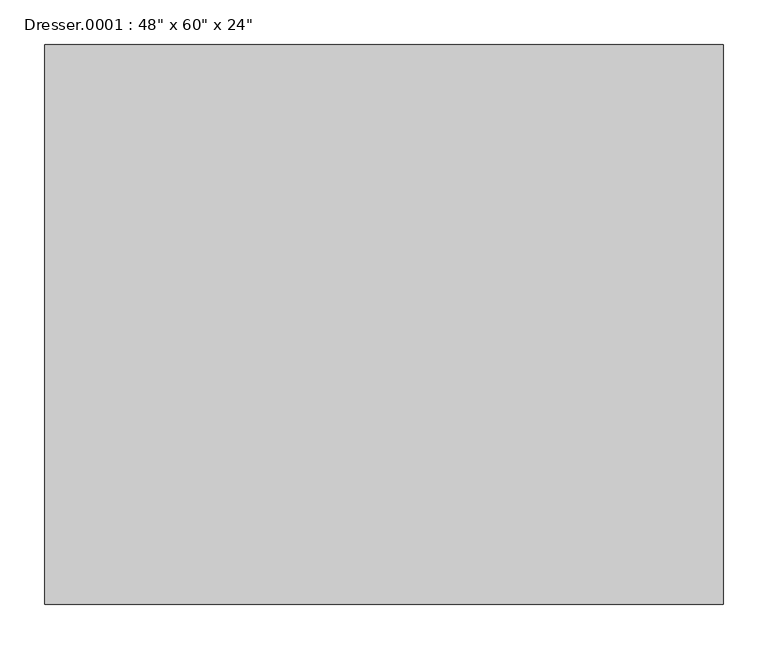
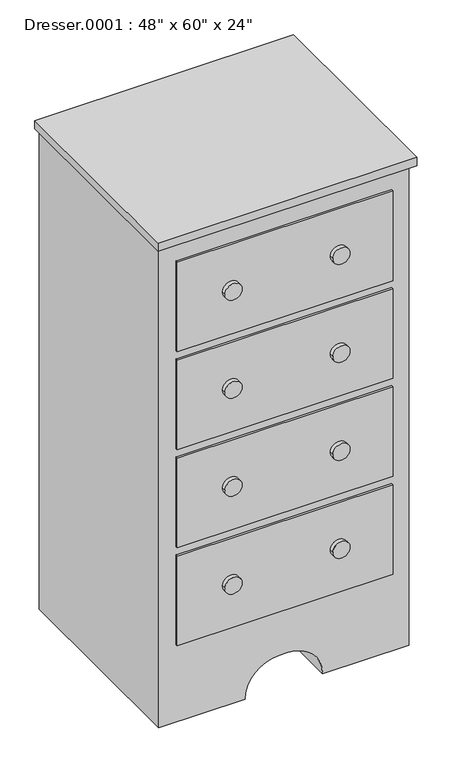
"""IFC4 building model written with IfcOpenShell, lengths in millimetres: furniture geometry."""

from ifc_helpers import new_model, si_unit, point, frame, frame_2d, origin, place, context, project, spatial, polyline, circle_curve, trimmed, segment, composite_curve, outline, extrude, source, transform, mapped, element, save


def furniture_08c10487(model_context):
    return source(origin(), model_context, "Body", "SweptSolid", [
        extrude(outline(polyline([(111.8067402, -58.3629541), (111.8067402, -687.0129541), (-650.1932598, -687.0129541), (-650.1932598, -58.3629541), (111.8067402, -58.3629541)])), frame((0.0, 0.0, 1498.6), z_axis=(0.0, 0.0, 1.0), x_axis=(1.0, 0.0, 0.0)), (0.0, 0.0, 1.0), 25.4),
        extrude(outline(composite_curve([segment(polyline([(0.0, 99.1067402), (1498.6, 99.1067402), (1498.6, -637.4932598), (0.0, -637.4932598), (0.0, -383.4932598)]), True, "CONTINUOUS"), segment(trimmed(circle_curve(frame_2d((0.0, -281.8932598)), 101.6), [point((0.0, -383.4932598))], [point((101.6, -281.8932598))], True, "CARTESIAN"), True, "CONTINUOUS"), segment(polyline([(101.6, -281.8932598), (101.6, -256.4932598)]), True, "CONTINUOUS"), segment(trimmed(circle_curve(frame_2d((0.0, -256.4932598)), 101.6), [point((101.6, -256.4932598))], [point((0.0, -154.8932598))], True, "CARTESIAN"), True, "CONTINUOUS"), segment(polyline([(0.0, -154.8932598), (0.0, 99.1067402)]), True, "CONTINUOUS")], self_intersect=False)), frame((0.0, -667.9629541, 0.0), z_axis=(0.0, 1.0, 0.0), x_axis=(0.0, 0.0, 1.0)), (0.0, 0.0, 1.0), 609.6),
        extrude(outline(composite_curve([segment(trimmed(circle_curve(frame_2d((1295.4, -110.4432598)), 25.4), [point((1295.4, -135.8432598))], [point((1295.4, -85.0432598))], False, "CARTESIAN"), True, "CONTINUOUS"), segment(trimmed(circle_curve(frame_2d((1295.4, -110.4432598)), 25.4), [point((1295.4, -85.0432598))], [point((1295.4, -135.8432598))], False, "CARTESIAN"), True, "CONTINUOUS")], self_intersect=False)), frame((0.0, -687.0129541, 0.0), z_axis=(0.0, 1.0, 0.0), x_axis=(0.0, 0.0, 1.0)), (0.0, 0.0, 1.0), 12.7),
        extrude(outline(composite_curve([segment(trimmed(circle_curve(frame_2d((990.6, -110.4432598)), 25.4), [point((990.6, -135.8432598))], [point((990.6, -85.0432598))], False, "CARTESIAN"), True, "CONTINUOUS"), segment(trimmed(circle_curve(frame_2d((990.6, -110.4432598)), 25.4), [point((990.6, -85.0432598))], [point((990.6, -135.8432598))], False, "CARTESIAN"), True, "CONTINUOUS")], self_intersect=False)), frame((0.0, -687.0129541, 0.0), z_axis=(0.0, 1.0, 0.0), x_axis=(0.0, 0.0, 1.0)), (0.0, 0.0, 1.0), 12.7),
        extrude(outline(composite_curve([segment(trimmed(circle_curve(frame_2d((685.8, -110.4432598)), 25.4), [point((685.8, -135.8432598))], [point((685.8, -85.0432598))], False, "CARTESIAN"), True, "CONTINUOUS"), segment(trimmed(circle_curve(frame_2d((685.8, -110.4432598)), 25.4), [point((685.8, -85.0432598))], [point((685.8, -135.8432598))], False, "CARTESIAN"), True, "CONTINUOUS")], self_intersect=False)), frame((0.0, -687.0129541, 0.0), z_axis=(0.0, 1.0, 0.0), x_axis=(0.0, 0.0, 1.0)), (0.0, 0.0, 1.0), 12.7),
        extrude(outline(composite_curve([segment(trimmed(circle_curve(frame_2d((381.0, -110.4432598)), 25.4), [point((381.0, -135.8432598))], [point((381.0, -85.0432598))], False, "CARTESIAN"), True, "CONTINUOUS"), segment(trimmed(circle_curve(frame_2d((381.0, -110.4432598)), 25.4), [point((381.0, -85.0432598))], [point((381.0, -135.8432598))], False, "CARTESIAN"), True, "CONTINUOUS")], self_intersect=False)), frame((0.0, -687.0129541, 0.0), z_axis=(0.0, 1.0, 0.0), x_axis=(0.0, 0.0, 1.0)), (0.0, 0.0, 1.0), 12.7),
        extrude(outline(composite_curve([segment(trimmed(circle_curve(frame_2d((381.0, -427.9432598)), 25.4), [point((381.0, -453.3432598))], [point((381.0, -402.5432598))], False, "CARTESIAN"), True, "CONTINUOUS"), segment(trimmed(circle_curve(frame_2d((381.0, -427.9432598)), 25.4), [point((381.0, -402.5432598))], [point((381.0, -453.3432598))], False, "CARTESIAN"), True, "CONTINUOUS")], self_intersect=False)), frame((0.0, -687.0129541, 0.0), z_axis=(0.0, 1.0, 0.0), x_axis=(0.0, 0.0, 1.0)), (0.0, 0.0, 1.0), 12.7),
        extrude(outline(composite_curve([segment(trimmed(circle_curve(frame_2d((685.8, -427.9432598)), 25.4), [point((685.8, -453.3432598))], [point((685.8, -402.5432598))], False, "CARTESIAN"), True, "CONTINUOUS"), segment(trimmed(circle_curve(frame_2d((685.8, -427.9432598)), 25.4), [point((685.8, -402.5432598))], [point((685.8, -453.3432598))], False, "CARTESIAN"), True, "CONTINUOUS")], self_intersect=False)), frame((0.0, -687.0129541, 0.0), z_axis=(0.0, 1.0, 0.0), x_axis=(0.0, 0.0, 1.0)), (0.0, 0.0, 1.0), 12.7),
        extrude(outline(composite_curve([segment(trimmed(circle_curve(frame_2d((990.6, -427.9432598)), 25.4), [point((990.6, -453.3432598))], [point((990.6, -402.5432598))], False, "CARTESIAN"), True, "CONTINUOUS"), segment(trimmed(circle_curve(frame_2d((990.6, -427.9432598)), 25.4), [point((990.6, -402.5432598))], [point((990.6, -453.3432598))], False, "CARTESIAN"), True, "CONTINUOUS")], self_intersect=False)), frame((0.0, -687.0129541, 0.0), z_axis=(0.0, 1.0, 0.0), x_axis=(0.0, 0.0, 1.0)), (0.0, 0.0, 1.0), 12.7),
        extrude(outline(composite_curve([segment(trimmed(circle_curve(frame_2d((1295.4, -427.9432598)), 25.4), [point((1295.4, -453.3432598))], [point((1295.4, -402.5432598))], False, "CARTESIAN"), True, "CONTINUOUS"), segment(trimmed(circle_curve(frame_2d((1295.4, -427.9432598)), 25.4), [point((1295.4, -402.5432598))], [point((1295.4, -453.3432598))], False, "CARTESIAN"), True, "CONTINUOUS")], self_intersect=False)), frame((0.0, -687.0129541, 0.0), z_axis=(0.0, 1.0, 0.0), x_axis=(0.0, 0.0, 1.0)), (0.0, 0.0, 1.0), 12.7),
        extrude(outline(polyline([(48.3067402, -674.3129541), (-586.6932598, -674.3129541), (-586.6932598, -667.9629541), (48.3067402, -667.9629541), (48.3067402, -674.3129541)])), frame((0.0, 0.0, 1155.7), z_axis=(0.0, 0.0, 1.0), x_axis=(1.0, 0.0, 0.0)), (0.0, 0.0, 1.0), 279.4),
        extrude(outline(polyline([(48.3067402, -674.3129541), (-586.6932598, -674.3129541), (-586.6932598, -667.9629541), (48.3067402, -667.9629541), (48.3067402, -674.3129541)])), frame((0.0, 0.0, 850.9), z_axis=(0.0, 0.0, 1.0), x_axis=(1.0, 0.0, 0.0)), (0.0, 0.0, 1.0), 279.4),
        extrude(outline(polyline([(48.3067402, -674.3129541), (-586.6932598, -674.3129541), (-586.6932598, -667.9629541), (48.3067402, -667.9629541), (48.3067402, -674.3129541)])), frame((0.0, 0.0, 546.1), z_axis=(0.0, 0.0, 1.0), x_axis=(1.0, 0.0, 0.0)), (0.0, 0.0, 1.0), 279.4),
        extrude(outline(polyline([(48.3067402, -674.3129541), (-586.6932598, -674.3129541), (-586.6932598, -667.9629541), (48.3067402, -667.9629541), (48.3067402, -674.3129541)])), frame((0.0, 0.0, 241.3), z_axis=(0.0, 0.0, 1.0), x_axis=(1.0, 0.0, 0.0)), (0.0, 0.0, 1.0), 279.4),
    ])


if __name__ == "__main__":
    model = new_model("IFC4")
    model_context = context("Model", 3, world=origin())
    ifc_project = project(units=[si_unit("LENGTHUNIT", "METRE", prefix="MILLI")], contexts=[model_context])
    site = spatial("IfcSite", under=ifc_project)
    building = spatial("IfcBuilding", under=site)
    placement = place(None, origin())
    furniture_shape = furniture_08c10487(model_context)
    element("IfcFurniture", 1, ObjectType="Dresser.0001 : 48\" x 60\" x 24\"", at=placement, inside=building, context=model_context, shape_type="MappedRepresentation", body=[
        mapped(furniture_shape, transform((0.0, 0.0, 0.0), x_axis=(1.0, 0.0, 0.0), y_axis=(0.0, 1.0, 0.0), z_axis=(0.0, 0.0, 1.0))),
    ])
    save(model, "model.ifc")

# Revit data of these elements
# Type "Dresser.0001 : 48\" x 60\" x 24\""
#   Assembly Code = "E2020200"
#   Depth = 2' - 0"
#   Height = 5' - 0"
#   Width = 2' - 5"
#   Dresser Material = Laminate - Ivory, Glossy
#   Drawer Material = Laminate, Ivory, Matte
#   Knob Material = Cherry
#   Default Elevation = 0
# Element 1 (IfcFurniture, "Dresser.0001 : 48\" x 60\" x 24\"")
#   Materials on its faces: "Laminate, Ivory, Matte", "Cherry", "Laminate - Ivory, Glossy"
# Materials
#   "Laminate - Ivory, Glossy": colour RGB 247 247 239, transparency 0
#   "Laminate, Ivory, Matte": class "Plastic", colour RGB 247 247 239, transparency 0, Description = "Plastic Laminate - Ivory, Matte", Cost = 0
#   "Cherry": class "Wood", colour RGB 226 177 128, transparency 0, Description = "Prunus Serotina", Cost = 0
